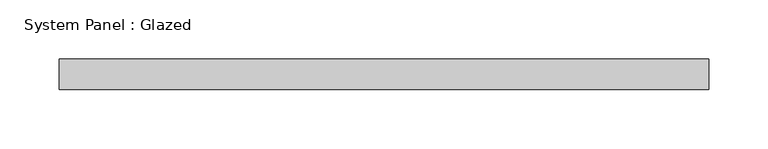
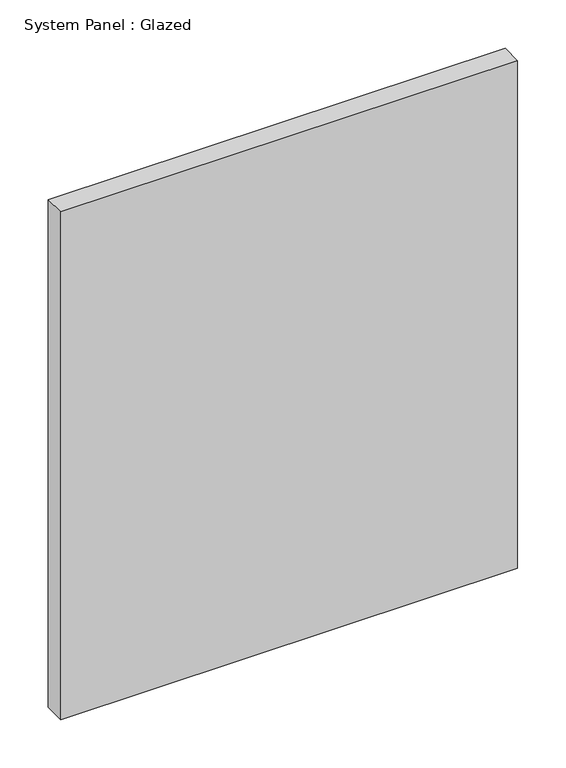
"""IFC4 building model written with IfcOpenShell, lengths in millimetres: plate geometry, System Panel : Glazed."""

from ifc_helpers import new_model, si_unit, origin, origin_with_axes, place, context, project, spatial, polyline, outline, extrude, source, transform, mapped, element, save


def system_panel_glazed_56d4eafa(model_context):
    return source(origin(), model_context, "Body", "SweptSolid", [
        extrude(outline(polyline([(273.05, 19.05), (-273.05, 19.05), (-273.05, 44.45), (273.05, 44.45), (273.05, 19.05)])), origin_with_axes(), (0.0, 0.0, 1.0), 641.0467564),
    ])


if __name__ == "__main__":
    model = new_model("IFC4")
    model_context = context("Model", 3, world=origin())
    ifc_project = project(units=[si_unit("LENGTHUNIT", "METRE", prefix="MILLI")], contexts=[model_context])
    site = spatial("IfcSite", under=ifc_project)
    building = spatial("IfcBuilding", under=site)
    placement = place(None, origin())
    system_panel_glazed_shape = system_panel_glazed_56d4eafa(model_context)
    element("IfcPlate", 1, ObjectType="System Panel : Glazed", at=placement, inside=building, context=model_context, shape_type="MappedRepresentation", body=[
        mapped(system_panel_glazed_shape, transform((0.0, 0.0, 0.0), x_axis=(1.0, 0.0, 0.0), y_axis=(0.0, 1.0, 0.0), z_axis=(0.0, 0.0, 1.0))),
    ])
    save(model, "model.ifc")

# Revit data of these elements
# Type "System Panel : Glazed"
#   Construction Type Id = "GSP4R"
#   Analytic Construction = "1/8 in Pilkington single glazing"
#   Visual Light Transmittance = 0.9
#   Solar Heat Gain Coefficient = 0.86
#   Heat Transfer Coefficient (U) = 1.18115 BTU/(h·ft²·°F)
#   Define Thermal Properties by = 1
# Element 1 (IfcPlate, "System Panel : Glazed")
#   Materials on its faces: "Glass"
# Materials
#   "Glass": class "Glass", colour RGB 0 128 192, transparency 0.75, Description = "Soda Lime Glass", Cost = 0
